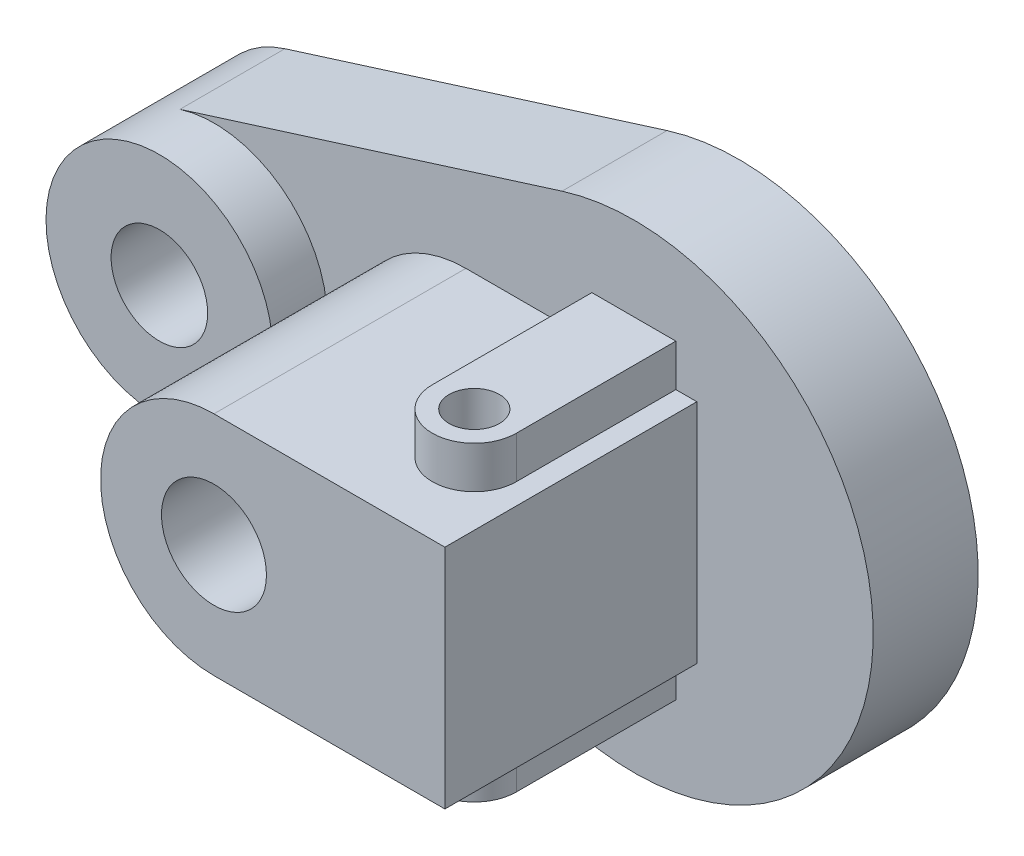
ISO-10303-21;
HEADER;
FILE_DESCRIPTION(('STEP AP214'),'2;1');
FILE_NAME('part.step','',(''),(''),'','','');
FILE_SCHEMA(('AUTOMOTIVE_DESIGN { 1 0 10303 214 1 1 1 1 }'));
ENDSEC;
DATA;
#1=APPLICATION_CONTEXT('core data for automotive mechanical design processes');
#2=APPLICATION_PROTOCOL_DEFINITION('international standard','automotive_design',2000,#1);
#3=PRODUCT_CONTEXT('',#1,'mechanical');
#4=PRODUCT('Part','Part','',(#3));
#5=PRODUCT_RELATED_PRODUCT_CATEGORY('part','',(#4));
#6=PRODUCT_DEFINITION_FORMATION('','',#4);
#7=PRODUCT_DEFINITION_CONTEXT('part definition',#1,'design');
#8=PRODUCT_DEFINITION('design','',#6,#7);
#9=PRODUCT_DEFINITION_SHAPE('','',#8);
#10=(LENGTH_UNIT() NAMED_UNIT(*) SI_UNIT(.MILLI.,.METRE.));
#11=(NAMED_UNIT(*) PLANE_ANGLE_UNIT() SI_UNIT($,.RADIAN.));
#12=(NAMED_UNIT(*) SI_UNIT($,.STERADIAN.) SOLID_ANGLE_UNIT());
#13=UNCERTAINTY_MEASURE_WITH_UNIT(LENGTH_MEASURE(1.E-05),#10,'distance_accuracy_value','');
#14=(GEOMETRIC_REPRESENTATION_CONTEXT(3) GLOBAL_UNCERTAINTY_ASSIGNED_CONTEXT((#13)) GLOBAL_UNIT_ASSIGNED_CONTEXT((#10,
#11,#12)) REPRESENTATION_CONTEXT('',''));
#15=CARTESIAN_POINT('',(0.,0.,0.));
#16=DIRECTION('',(0.,0.,1.));
#17=DIRECTION('',(1.,0.,0.));
#18=AXIS2_PLACEMENT_3D('',#15,#16,#17);
#19=CARTESIAN_POINT('',(0.,0.,25.));
#20=DIRECTION('',(0.,0.,1.));
#21=DIRECTION('',(1.,0.,0.));
#22=AXIS2_PLACEMENT_3D('',#19,#20,#21);
#23=PLANE('',#22);
#24=DIRECTION('',(0.,-1.,0.));
#25=VECTOR('',#24,1.);
#26=CARTESIAN_POINT('',(110.,37.,25.));
#27=LINE('',#26,#25);
#28=CARTESIAN_POINT('',(110.,37.,25.));
#29=VERTEX_POINT('',#28);
#30=CARTESIAN_POINT('',(110.,27.,25.));
#31=VERTEX_POINT('',#30);
#32=EDGE_CURVE('E164',#29,#31,#27,.T.);
#33=ORIENTED_EDGE('',*,*,#32,.T.);
#34=DIRECTION('',(-1.,0.,0.));
#35=VECTOR('',#34,1.);
#36=CARTESIAN_POINT('',(60.,27.,25.));
#37=LINE('',#36,#35);
#38=CARTESIAN_POINT('',(115.,27.,25.));
#39=VERTEX_POINT('',#38);
#40=EDGE_CURVE('E237',#39,#31,#37,.T.);
#41=ORIENTED_EDGE('',*,*,#40,.F.);
#42=DIRECTION('',(0.,1.,0.));
#43=VECTOR('',#42,1.);
#44=CARTESIAN_POINT('',(115.,27.,25.));
#45=LINE('',#44,#43);
#46=CARTESIAN_POINT('',(115.,-27.,25.));
#47=VERTEX_POINT('',#46);
#48=EDGE_CURVE('E248',#47,#39,#45,.T.);
#49=ORIENTED_EDGE('',*,*,#48,.F.);
#50=DIRECTION('',(1.,0.,0.));
#51=VECTOR('',#50,1.);
#52=CARTESIAN_POINT('',(115.,-27.,25.));
#53=LINE('',#52,#51);
#54=CARTESIAN_POINT('',(110.,-27.,25.));
#55=VERTEX_POINT('',#54);
#56=EDGE_CURVE('E242',#55,#47,#53,.T.);
#57=ORIENTED_EDGE('',*,*,#56,.F.);
#58=DIRECTION('',(0.,1.,0.));
#59=VECTOR('',#58,1.);
#60=CARTESIAN_POINT('',(110.,-37.,25.));
#61=LINE('',#60,#59);
#62=CARTESIAN_POINT('',(110.,-37.,25.));
#63=VERTEX_POINT('',#62);
#64=EDGE_CURVE('E220',#63,#55,#61,.T.);
#65=ORIENTED_EDGE('',*,*,#64,.F.);
#66=DIRECTION('',(1.,0.,0.));
#67=VECTOR('',#66,1.);
#68=CARTESIAN_POINT('',(90.,-37.,25.));
#69=LINE('',#68,#67);
#70=CARTESIAN_POINT('',(90.,-37.,25.));
#71=VERTEX_POINT('',#70);
#72=EDGE_CURVE('E65',#71,#63,#69,.T.);
#73=ORIENTED_EDGE('',*,*,#72,.F.);
#74=DIRECTION('',(0.,1.,0.));
#75=VECTOR('',#74,1.);
#76=CARTESIAN_POINT('',(90.,-37.,25.));
#77=LINE('',#76,#75);
#78=CARTESIAN_POINT('',(90.,-27.,25.));
#79=VERTEX_POINT('',#78);
#80=EDGE_CURVE('E219',#71,#79,#77,.T.);
#81=ORIENTED_EDGE('',*,*,#80,.T.);
#82=CARTESIAN_POINT('',(60.,-27.,25.));
#83=VERTEX_POINT('',#82);
#84=EDGE_CURVE('E246',#83,#79,#53,.T.);
#85=ORIENTED_EDGE('',*,*,#84,.F.);
#86=CARTESIAN_POINT('',(60.,0.,25.));
#87=DIRECTION('',(0.,0.,1.));
#88=DIRECTION('',(1.,0.,0.));
#89=AXIS2_PLACEMENT_3D('',#86,#87,#88);
#90=CIRCLE('',#89,27.);
#91=CARTESIAN_POINT('',(60.,27.,25.));
#92=VERTEX_POINT('',#91);
#93=EDGE_CURVE('E229',#92,#83,#90,.T.);
#94=ORIENTED_EDGE('',*,*,#93,.F.);
#95=CARTESIAN_POINT('',(90.,27.,25.));
#96=VERTEX_POINT('',#95);
#97=EDGE_CURVE('E252',#96,#92,#37,.T.);
#98=ORIENTED_EDGE('',*,*,#97,.F.);
#99=DIRECTION('',(0.,-1.,0.));
#100=VECTOR('',#99,1.);
#101=CARTESIAN_POINT('',(90.,37.,25.));
#102=LINE('',#101,#100);
#103=CARTESIAN_POINT('',(90.,37.,25.));
#104=VERTEX_POINT('',#103);
#105=EDGE_CURVE('E53',#104,#96,#102,.T.);
#106=ORIENTED_EDGE('',*,*,#105,.F.);
#107=DIRECTION('',(1.,0.,0.));
#108=VECTOR('',#107,1.);
#109=CARTESIAN_POINT('',(90.,37.,25.));
#110=LINE('',#109,#108);
#111=EDGE_CURVE('E180',#104,#29,#110,.T.);
#112=ORIENTED_EDGE('',*,*,#111,.T.);
#113=EDGE_LOOP('',(#33,#41,#49,#57,#65,#73,#81,#85,#94,#98,#106,#112));
#114=FACE_BOUND('',#113,.T.);
#115=CARTESIAN_POINT('',(0.,0.,25.));
#116=DIRECTION('',(0.,0.,-1.));
#117=DIRECTION('',(1.,0.,0.));
#118=AXIS2_PLACEMENT_3D('',#115,#116,#117);
#119=CIRCLE('',#118,27.);
#120=CARTESIAN_POINT('',(-8.1,25.7563584382575,25.));
#121=VERTEX_POINT('',#120);
#122=CARTESIAN_POINT('',(-8.1,-25.7563584382575,25.));
#123=VERTEX_POINT('',#122);
#124=EDGE_CURVE('E264',#121,#123,#119,.T.);
#125=ORIENTED_EDGE('',*,*,#124,.T.);
#126=DIRECTION('',(0.953939201416946,-0.3,0.));
#127=VECTOR('',#126,1.);
#128=CARTESIAN_POINT('',(-8.1,-25.7563584382575,25.));
#129=LINE('',#128,#127);
#130=CARTESIAN_POINT('',(82.9,-54.3745344807659,25.));
#131=VERTEX_POINT('',#130);
#132=EDGE_CURVE('E268',#123,#131,#129,.T.);
#133=ORIENTED_EDGE('',*,*,#132,.T.);
#134=CARTESIAN_POINT('',(100.,0.,25.));
#135=DIRECTION('',(0.,0.,1.));
#136=DIRECTION('',(1.,0.,0.));
#137=AXIS2_PLACEMENT_3D('',#134,#135,#136);
#138=CIRCLE('',#137,57.);
#139=CARTESIAN_POINT('',(82.9,54.3745344807659,25.));
#140=VERTEX_POINT('',#139);
#141=EDGE_CURVE('E271',#131,#140,#138,.T.);
#142=ORIENTED_EDGE('',*,*,#141,.T.);
#143=DIRECTION('',(-0.953939201416946,-0.3,0.));
#144=VECTOR('',#143,1.);
#145=CARTESIAN_POINT('',(-8.1,25.7563584382575,25.));
#146=LINE('',#145,#144);
#147=EDGE_CURVE('E272',#140,#121,#146,.T.);
#148=ORIENTED_EDGE('',*,*,#147,.T.);
#149=EDGE_LOOP('',(#125,#133,#142,#148));
#150=FACE_BOUND('',#149,.T.);
#151=ADVANCED_FACE('F39',(#114,#150),#23,.T.);
#152=CARTESIAN_POINT('',(0.,0.,38.));
#153=DIRECTION('',(0.,0.,-1.));
#154=DIRECTION('',(-1.,0.,0.));
#155=AXIS2_PLACEMENT_3D('',#152,#153,#154);
#156=CYLINDRICAL_SURFACE('',#155,27.);
#157=CARTESIAN_POINT('',(0.,0.,38.));
#158=DIRECTION('',(0.,0.,1.));
#159=DIRECTION('',(1.,0.,0.));
#160=AXIS2_PLACEMENT_3D('',#157,#158,#159);
#161=CIRCLE('',#160,27.);
#162=CARTESIAN_POINT('',(27.,0.,38.));
#163=VERTEX_POINT('',#162);
#164=EDGE_CURVE('E50',#163,#163,#161,.T.);
#165=ORIENTED_EDGE('',*,*,#164,.F.);
#166=EDGE_LOOP('',(#165));
#167=FACE_BOUND('',#166,.T.);
#168=DIRECTION('',(0.,0.,-1.));
#169=VECTOR('',#168,1.);
#170=CARTESIAN_POINT('',(-8.1,-25.7563584382575,25.));
#171=LINE('',#170,#169);
#172=CARTESIAN_POINT('',(-8.1,-25.7563584382575,0.));
#173=VERTEX_POINT('',#172);
#174=EDGE_CURVE('E289',#123,#173,#171,.T.);
#175=ORIENTED_EDGE('',*,*,#174,.F.);
#176=ORIENTED_EDGE('',*,*,#124,.F.);
#177=DIRECTION('',(0.,0.,-1.));
#178=VECTOR('',#177,1.);
#179=CARTESIAN_POINT('',(-8.1,25.7563584382575,25.));
#180=LINE('',#179,#178);
#181=CARTESIAN_POINT('',(-8.1,25.7563584382575,0.));
#182=VERTEX_POINT('',#181);
#183=EDGE_CURVE('E277',#121,#182,#180,.T.);
#184=ORIENTED_EDGE('',*,*,#183,.T.);
#185=CARTESIAN_POINT('',(0.,0.,0.));
#186=DIRECTION('',(0.,0.,1.));
#187=DIRECTION('',(1.,0.,0.));
#188=AXIS2_PLACEMENT_3D('',#185,#186,#187);
#189=CIRCLE('',#188,27.);
#190=EDGE_CURVE('E300',#182,#173,#189,.T.);
#191=ORIENTED_EDGE('',*,*,#190,.T.);
#192=EDGE_LOOP('',(#175,#176,#184,#191));
#193=FACE_BOUND('',#192,.T.);
#194=ADVANCED_FACE('F41',(#167,#193),#156,.T.);
#195=CARTESIAN_POINT('',(0.,0.,38.));
#196=DIRECTION('',(0.,0.,1.));
#197=DIRECTION('',(1.,0.,0.));
#198=AXIS2_PLACEMENT_3D('',#195,#196,#197);
#199=PLANE('',#198);
#200=ORIENTED_EDGE('',*,*,#164,.T.);
#201=EDGE_LOOP('',(#200));
#202=FACE_BOUND('',#201,.T.);
#203=CARTESIAN_POINT('',(0.,0.,38.));
#204=DIRECTION('',(0.,0.,1.));
#205=DIRECTION('',(1.,0.,0.));
#206=AXIS2_PLACEMENT_3D('',#203,#204,#205);
#207=CIRCLE('',#206,11.5);
#208=CARTESIAN_POINT('',(11.5,0.,38.));
#209=VERTEX_POINT('',#208);
#210=EDGE_CURVE('E294',#209,#209,#207,.T.);
#211=ORIENTED_EDGE('',*,*,#210,.F.);
#212=EDGE_LOOP('',(#211));
#213=FACE_BOUND('',#212,.T.);
#214=ADVANCED_FACE('F336',(#202,#213),#199,.T.);
#215=CARTESIAN_POINT('',(0.,0.,0.));
#216=DIRECTION('',(0.,0.,1.));
#217=DIRECTION('',(1.,0.,0.));
#218=AXIS2_PLACEMENT_3D('',#215,#216,#217);
#219=PLANE('',#218);
#220=ORIENTED_EDGE('',*,*,#190,.F.);
#221=DIRECTION('',(-0.953939201416946,-0.3,0.));
#222=VECTOR('',#221,1.);
#223=CARTESIAN_POINT('',(-8.1,25.7563584382575,0.));
#224=LINE('',#223,#222);
#225=CARTESIAN_POINT('',(82.9,54.3745344807659,0.));
#226=VERTEX_POINT('',#225);
#227=EDGE_CURVE('E267',#226,#182,#224,.T.);
#228=ORIENTED_EDGE('',*,*,#227,.F.);
#229=CARTESIAN_POINT('',(100.,0.,0.));
#230=DIRECTION('',(0.,0.,1.));
#231=DIRECTION('',(1.,0.,0.));
#232=AXIS2_PLACEMENT_3D('',#229,#230,#231);
#233=CIRCLE('',#232,57.);
#234=CARTESIAN_POINT('',(82.9,-54.3745344807659,0.));
#235=VERTEX_POINT('',#234);
#236=EDGE_CURVE('E279',#235,#226,#233,.T.);
#237=ORIENTED_EDGE('',*,*,#236,.F.);
#238=DIRECTION('',(0.953939201416946,-0.3,0.));
#239=VECTOR('',#238,1.);
#240=CARTESIAN_POINT('',(-8.1,-25.7563584382575,0.));
#241=LINE('',#240,#239);
#242=EDGE_CURVE('E262',#173,#235,#241,.T.);
#243=ORIENTED_EDGE('',*,*,#242,.F.);
#244=EDGE_LOOP('',(#220,#228,#237,#243));
#245=FACE_BOUND('',#244,.T.);
#246=CARTESIAN_POINT('',(0.,0.,0.));
#247=DIRECTION('',(0.,0.,1.));
#248=DIRECTION('',(1.,0.,0.));
#249=AXIS2_PLACEMENT_3D('',#246,#247,#248);
#250=CIRCLE('',#249,11.5);
#251=CARTESIAN_POINT('',(11.5,0.,0.));
#252=VERTEX_POINT('',#251);
#253=EDGE_CURVE('E291',#252,#252,#250,.T.);
#254=ORIENTED_EDGE('',*,*,#253,.T.);
#255=EDGE_LOOP('',(#254));
#256=FACE_BOUND('',#255,.T.);
#257=ADVANCED_FACE('F306',(#245,#256),#219,.F.);
#258=CARTESIAN_POINT('',(0.,0.,38.));
#259=DIRECTION('',(0.,0.,-1.));
#260=DIRECTION('',(-1.,0.,0.));
#261=AXIS2_PLACEMENT_3D('',#258,#259,#260);
#262=CYLINDRICAL_SURFACE('',#261,11.5);
#263=ORIENTED_EDGE('',*,*,#210,.T.);
#264=EDGE_LOOP('',(#263));
#265=FACE_BOUND('',#264,.T.);
#266=ORIENTED_EDGE('',*,*,#253,.F.);
#267=EDGE_LOOP('',(#266));
#268=FACE_BOUND('',#267,.T.);
#269=ADVANCED_FACE('F328',(#265,#268),#262,.F.);
#270=CARTESIAN_POINT('',(-8.1,-25.7563584382575,25.));
#271=DIRECTION('',(0.3,0.953939201416946,0.));
#272=DIRECTION('',(-0.953939201416946,0.3,0.));
#273=AXIS2_PLACEMENT_3D('',#270,#271,#272);
#274=PLANE('',#273);
#275=ORIENTED_EDGE('',*,*,#242,.T.);
#276=DIRECTION('',(0.,0.,-1.));
#277=VECTOR('',#276,1.);
#278=CARTESIAN_POINT('',(82.9,-54.3745344807659,25.));
#279=LINE('',#278,#277);
#280=EDGE_CURVE('E290',#131,#235,#279,.T.);
#281=ORIENTED_EDGE('',*,*,#280,.F.);
#282=ORIENTED_EDGE('',*,*,#132,.F.);
#283=ORIENTED_EDGE('',*,*,#174,.T.);
#284=EDGE_LOOP('',(#275,#281,#282,#283));
#285=FACE_BOUND('',#284,.T.);
#286=ADVANCED_FACE('F315',(#285),#274,.F.);
#287=CARTESIAN_POINT('',(100.,0.,25.));
#288=DIRECTION('',(0.,0.,-1.));
#289=DIRECTION('',(-1.,0.,0.));
#290=AXIS2_PLACEMENT_3D('',#287,#288,#289);
#291=CYLINDRICAL_SURFACE('',#290,57.);
#292=ORIENTED_EDGE('',*,*,#236,.T.);
#293=DIRECTION('',(0.,0.,-1.));
#294=VECTOR('',#293,1.);
#295=CARTESIAN_POINT('',(82.9,54.3745344807659,25.));
#296=LINE('',#295,#294);
#297=EDGE_CURVE('E284',#140,#226,#296,.T.);
#298=ORIENTED_EDGE('',*,*,#297,.F.);
#299=ORIENTED_EDGE('',*,*,#141,.F.);
#300=ORIENTED_EDGE('',*,*,#280,.T.);
#301=EDGE_LOOP('',(#292,#298,#299,#300));
#302=FACE_BOUND('',#301,.T.);
#303=ADVANCED_FACE('F319',(#302),#291,.T.);
#304=CARTESIAN_POINT('',(-8.1,25.7563584382575,25.));
#305=DIRECTION('',(0.3,-0.953939201416946,0.));
#306=DIRECTION('',(0.953939201416946,0.3,0.));
#307=AXIS2_PLACEMENT_3D('',#304,#305,#306);
#308=PLANE('',#307);
#309=ORIENTED_EDGE('',*,*,#227,.T.);
#310=ORIENTED_EDGE('',*,*,#183,.F.);
#311=ORIENTED_EDGE('',*,*,#147,.F.);
#312=ORIENTED_EDGE('',*,*,#297,.T.);
#313=EDGE_LOOP('',(#309,#310,#311,#312));
#314=FACE_BOUND('',#313,.T.);
#315=ADVANCED_FACE('F318',(#314),#308,.F.);
#316=CARTESIAN_POINT('',(60.,0.,85.));
#317=DIRECTION('',(0.,0.,-1.));
#318=DIRECTION('',(-1.,0.,0.));
#319=AXIS2_PLACEMENT_3D('',#316,#317,#318);
#320=CYLINDRICAL_SURFACE('',#319,27.);
#321=ORIENTED_EDGE('',*,*,#93,.T.);
#322=DIRECTION('',(0.,0.,-1.));
#323=VECTOR('',#322,1.);
#324=CARTESIAN_POINT('',(60.,-27.,85.));
#325=LINE('',#324,#323);
#326=CARTESIAN_POINT('',(60.,-27.,85.));
#327=VERTEX_POINT('',#326);
#328=EDGE_CURVE('E265',#327,#83,#325,.T.);
#329=ORIENTED_EDGE('',*,*,#328,.F.);
#330=CARTESIAN_POINT('',(60.,0.,85.));
#331=DIRECTION('',(0.,0.,1.));
#332=DIRECTION('',(1.,0.,0.));
#333=AXIS2_PLACEMENT_3D('',#330,#331,#332);
#334=CIRCLE('',#333,27.);
#335=CARTESIAN_POINT('',(60.,27.,85.));
#336=VERTEX_POINT('',#335);
#337=EDGE_CURVE('E235',#336,#327,#334,.T.);
#338=ORIENTED_EDGE('',*,*,#337,.F.);
#339=DIRECTION('',(0.,0.,-1.));
#340=VECTOR('',#339,1.);
#341=CARTESIAN_POINT('',(60.,27.,85.));
#342=LINE('',#341,#340);
#343=EDGE_CURVE('E245',#336,#92,#342,.T.);
#344=ORIENTED_EDGE('',*,*,#343,.T.);
#345=EDGE_LOOP('',(#321,#329,#338,#344));
#346=FACE_BOUND('',#345,.T.);
#347=ADVANCED_FACE('F330',(#346),#320,.T.);
#348=CARTESIAN_POINT('',(115.,-27.,85.));
#349=DIRECTION('',(0.,1.,0.));
#350=DIRECTION('',(0.,0.,1.));
#351=AXIS2_PLACEMENT_3D('',#348,#349,#350);
#352=PLANE('',#351);
#353=DIRECTION('',(0.,0.,-1.));
#354=VECTOR('',#353,1.);
#355=CARTESIAN_POINT('',(90.,-27.,63.));
#356=LINE('',#355,#354);
#357=CARTESIAN_POINT('',(90.,-27.,63.));
#358=VERTEX_POINT('',#357);
#359=EDGE_CURVE('E209',#358,#79,#356,.T.);
#360=ORIENTED_EDGE('',*,*,#359,.F.);
#361=CARTESIAN_POINT('',(100.,-27.,63.));
#362=DIRECTION('',(0.,-1.,0.));
#363=DIRECTION('',(0.,0.,-1.));
#364=AXIS2_PLACEMENT_3D('',#361,#362,#363);
#365=CIRCLE('',#364,10.);
#366=CARTESIAN_POINT('',(110.,-27.,63.));
#367=VERTEX_POINT('',#366);
#368=EDGE_CURVE('E194',#367,#358,#365,.T.);
#369=ORIENTED_EDGE('',*,*,#368,.F.);
#370=DIRECTION('',(0.,0.,1.));
#371=VECTOR('',#370,1.);
#372=CARTESIAN_POINT('',(110.,-27.,25.));
#373=LINE('',#372,#371);
#374=EDGE_CURVE('E205',#55,#367,#373,.T.);
#375=ORIENTED_EDGE('',*,*,#374,.F.);
#376=ORIENTED_EDGE('',*,*,#56,.T.);
#377=DIRECTION('',(0.,0.,-1.));
#378=VECTOR('',#377,1.);
#379=CARTESIAN_POINT('',(115.,-27.,85.));
#380=LINE('',#379,#378);
#381=CARTESIAN_POINT('',(115.,-27.,85.));
#382=VERTEX_POINT('',#381);
#383=EDGE_CURVE('E259',#382,#47,#380,.T.);
#384=ORIENTED_EDGE('',*,*,#383,.F.);
#385=DIRECTION('',(1.,0.,0.));
#386=VECTOR('',#385,1.);
#387=CARTESIAN_POINT('',(115.,-27.,85.));
#388=LINE('',#387,#386);
#389=EDGE_CURVE('E234',#327,#382,#388,.T.);
#390=ORIENTED_EDGE('',*,*,#389,.F.);
#391=ORIENTED_EDGE('',*,*,#328,.T.);
#392=ORIENTED_EDGE('',*,*,#84,.T.);
#393=EDGE_LOOP('',(#360,#369,#375,#376,#384,#390,#391,#392));
#394=FACE_BOUND('',#393,.T.);
#395=ADVANCED_FACE('F342',(#394),#352,.F.);
#396=CARTESIAN_POINT('',(115.,27.,85.));
#397=DIRECTION('',(-1.,0.,0.));
#398=DIRECTION('',(0.,0.,1.));
#399=AXIS2_PLACEMENT_3D('',#396,#397,#398);
#400=PLANE('',#399);
#401=ORIENTED_EDGE('',*,*,#48,.T.);
#402=DIRECTION('',(0.,0.,-1.));
#403=VECTOR('',#402,1.);
#404=CARTESIAN_POINT('',(115.,27.,85.));
#405=LINE('',#404,#403);
#406=CARTESIAN_POINT('',(115.,27.,85.));
#407=VERTEX_POINT('',#406);
#408=EDGE_CURVE('E260',#407,#39,#405,.T.);
#409=ORIENTED_EDGE('',*,*,#408,.F.);
#410=DIRECTION('',(0.,1.,0.));
#411=VECTOR('',#410,1.);
#412=CARTESIAN_POINT('',(115.,27.,85.));
#413=LINE('',#412,#411);
#414=EDGE_CURVE('E236',#382,#407,#413,.T.);
#415=ORIENTED_EDGE('',*,*,#414,.F.);
#416=ORIENTED_EDGE('',*,*,#383,.T.);
#417=EDGE_LOOP('',(#401,#409,#415,#416));
#418=FACE_BOUND('',#417,.T.);
#419=ADVANCED_FACE('F350',(#418),#400,.F.);
#420=CARTESIAN_POINT('',(60.,27.,85.));
#421=DIRECTION('',(0.,-1.,0.));
#422=DIRECTION('',(0.,0.,-1.));
#423=AXIS2_PLACEMENT_3D('',#420,#421,#422);
#424=PLANE('',#423);
#425=ORIENTED_EDGE('',*,*,#40,.T.);
#426=DIRECTION('',(0.,0.,1.));
#427=VECTOR('',#426,1.);
#428=CARTESIAN_POINT('',(110.,27.,25.));
#429=LINE('',#428,#427);
#430=CARTESIAN_POINT('',(110.,27.,63.));
#431=VERTEX_POINT('',#430);
#432=EDGE_CURVE('E183',#31,#431,#429,.T.);
#433=ORIENTED_EDGE('',*,*,#432,.T.);
#434=CARTESIAN_POINT('',(100.,27.,63.));
#435=DIRECTION('',(0.,-1.,0.));
#436=DIRECTION('',(0.,0.,-1.));
#437=AXIS2_PLACEMENT_3D('',#434,#435,#436);
#438=CIRCLE('',#437,10.);
#439=CARTESIAN_POINT('',(90.,27.,63.));
#440=VERTEX_POINT('',#439);
#441=EDGE_CURVE('E159',#431,#440,#438,.T.);
#442=ORIENTED_EDGE('',*,*,#441,.T.);
#443=DIRECTION('',(0.,0.,-1.));
#444=VECTOR('',#443,1.);
#445=CARTESIAN_POINT('',(90.,27.,63.));
#446=LINE('',#445,#444);
#447=EDGE_CURVE('E171',#440,#96,#446,.T.);
#448=ORIENTED_EDGE('',*,*,#447,.T.);
#449=ORIENTED_EDGE('',*,*,#97,.T.);
#450=ORIENTED_EDGE('',*,*,#343,.F.);
#451=DIRECTION('',(-1.,0.,0.));
#452=VECTOR('',#451,1.);
#453=CARTESIAN_POINT('',(60.,27.,85.));
#454=LINE('',#453,#452);
#455=EDGE_CURVE('E238',#407,#336,#454,.T.);
#456=ORIENTED_EDGE('',*,*,#455,.F.);
#457=ORIENTED_EDGE('',*,*,#408,.T.);
#458=EDGE_LOOP('',(#425,#433,#442,#448,#449,#450,#456,#457));
#459=FACE_BOUND('',#458,.T.);
#460=ADVANCED_FACE('F355',(#459),#424,.F.);
#461=CARTESIAN_POINT('',(60.,0.,85.));
#462=DIRECTION('',(0.,0.,1.));
#463=DIRECTION('',(1.,0.,0.));
#464=AXIS2_PLACEMENT_3D('',#461,#462,#463);
#465=PLANE('',#464);
#466=CARTESIAN_POINT('',(60.,0.,85.));
#467=DIRECTION('',(0.,0.,1.));
#468=DIRECTION('',(1.,0.,0.));
#469=AXIS2_PLACEMENT_3D('',#466,#467,#468);
#470=CIRCLE('',#469,12.5);
#471=CARTESIAN_POINT('',(72.5,0.,85.));
#472=VERTEX_POINT('',#471);
#473=EDGE_CURVE('E223',#472,#472,#470,.T.);
#474=ORIENTED_EDGE('',*,*,#473,.F.);
#475=EDGE_LOOP('',(#474));
#476=FACE_BOUND('',#475,.T.);
#477=ORIENTED_EDGE('',*,*,#337,.T.);
#478=ORIENTED_EDGE('',*,*,#389,.T.);
#479=ORIENTED_EDGE('',*,*,#414,.T.);
#480=ORIENTED_EDGE('',*,*,#455,.T.);
#481=EDGE_LOOP('',(#477,#478,#479,#480));
#482=FACE_BOUND('',#481,.T.);
#483=ADVANCED_FACE('F352',(#476,#482),#465,.T.);
#484=CARTESIAN_POINT('',(60.,0.,25.));
#485=DIRECTION('',(0.,0.,1.));
#486=DIRECTION('',(1.,0.,0.));
#487=AXIS2_PLACEMENT_3D('',#484,#485,#486);
#488=CYLINDRICAL_SURFACE('',#487,12.5);
#489=CARTESIAN_POINT('',(60.,0.,25.));
#490=DIRECTION('',(0.,0.,1.));
#491=DIRECTION('',(1.,0.,0.));
#492=AXIS2_PLACEMENT_3D('',#489,#490,#491);
#493=CIRCLE('',#492,12.5);
#494=CARTESIAN_POINT('',(72.5,0.,25.));
#495=VERTEX_POINT('',#494);
#496=EDGE_CURVE('E228',#495,#495,#493,.T.);
#497=ORIENTED_EDGE('',*,*,#496,.F.);
#498=EDGE_LOOP('',(#497));
#499=FACE_BOUND('',#498,.T.);
#500=ORIENTED_EDGE('',*,*,#473,.T.);
#501=EDGE_LOOP('',(#500));
#502=FACE_BOUND('',#501,.T.);
#503=ADVANCED_FACE('F359',(#499,#502),#488,.F.);
#504=CARTESIAN_POINT('',(60.,0.,25.));
#505=DIRECTION('',(0.,0.,1.));
#506=DIRECTION('',(1.,0.,0.));
#507=AXIS2_PLACEMENT_3D('',#504,#505,#506);
#508=PLANE('',#507);
#509=ORIENTED_EDGE('',*,*,#496,.T.);
#510=EDGE_LOOP('',(#509));
#511=FACE_BOUND('',#510,.T.);
#512=ADVANCED_FACE('F365',(#511),#508,.T.);
#513=CARTESIAN_POINT('',(100.,-37.,63.));
#514=DIRECTION('',(0.,-1.,0.));
#515=DIRECTION('',(0.,0.,-1.));
#516=AXIS2_PLACEMENT_3D('',#513,#514,#515);
#517=PLANE('',#516);
#518=CARTESIAN_POINT('',(100.,-37.,63.));
#519=DIRECTION('',(0.,-1.,0.));
#520=DIRECTION('',(0.,0.,-1.));
#521=AXIS2_PLACEMENT_3D('',#518,#519,#520);
#522=CIRCLE('',#521,10.);
#523=CARTESIAN_POINT('',(110.,-37.,63.));
#524=VERTEX_POINT('',#523);
#525=CARTESIAN_POINT('',(90.,-37.,63.));
#526=VERTEX_POINT('',#525);
#527=EDGE_CURVE('E196',#524,#526,#522,.T.);
#528=ORIENTED_EDGE('',*,*,#527,.T.);
#529=DIRECTION('',(0.,0.,-1.));
#530=VECTOR('',#529,1.);
#531=CARTESIAN_POINT('',(90.,-37.,63.));
#532=LINE('',#531,#530);
#533=EDGE_CURVE('E203',#526,#71,#532,.T.);
#534=ORIENTED_EDGE('',*,*,#533,.T.);
#535=ORIENTED_EDGE('',*,*,#72,.T.);
#536=DIRECTION('',(0.,0.,1.));
#537=VECTOR('',#536,1.);
#538=CARTESIAN_POINT('',(110.,-37.,25.));
#539=LINE('',#538,#537);
#540=EDGE_CURVE('E202',#63,#524,#539,.T.);
#541=ORIENTED_EDGE('',*,*,#540,.T.);
#542=EDGE_LOOP('',(#528,#534,#535,#541));
#543=FACE_BOUND('',#542,.T.);
#544=CARTESIAN_POINT('',(100.,-37.,63.));
#545=DIRECTION('',(0.,-1.,0.));
#546=DIRECTION('',(0.,0.,-1.));
#547=AXIS2_PLACEMENT_3D('',#544,#545,#546);
#548=CIRCLE('',#547,6.);
#549=CARTESIAN_POINT('',(100.,-37.,57.));
#550=VERTEX_POINT('',#549);
#551=EDGE_CURVE('E195',#550,#550,#548,.T.);
#552=ORIENTED_EDGE('',*,*,#551,.F.);
#553=EDGE_LOOP('',(#552));
#554=FACE_BOUND('',#553,.T.);
#555=ADVANCED_FACE('F366',(#543,#554),#517,.T.);
#556=CARTESIAN_POINT('',(100.,-37.,63.));
#557=DIRECTION('',(0.,1.,0.));
#558=DIRECTION('',(0.,0.,1.));
#559=AXIS2_PLACEMENT_3D('',#556,#557,#558);
#560=CYLINDRICAL_SURFACE('',#559,10.);
#561=ORIENTED_EDGE('',*,*,#368,.T.);
#562=DIRECTION('',(0.,1.,0.));
#563=VECTOR('',#562,1.);
#564=CARTESIAN_POINT('',(90.,-37.,63.));
#565=LINE('',#564,#563);
#566=EDGE_CURVE('E225',#526,#358,#565,.T.);
#567=ORIENTED_EDGE('',*,*,#566,.F.);
#568=ORIENTED_EDGE('',*,*,#527,.F.);
#569=DIRECTION('',(0.,1.,0.));
#570=VECTOR('',#569,1.);
#571=CARTESIAN_POINT('',(110.,-37.,63.));
#572=LINE('',#571,#570);
#573=EDGE_CURVE('E210',#524,#367,#572,.T.);
#574=ORIENTED_EDGE('',*,*,#573,.T.);
#575=EDGE_LOOP('',(#561,#567,#568,#574));
#576=FACE_BOUND('',#575,.T.);
#577=ADVANCED_FACE('F367',(#576),#560,.T.);
#578=CARTESIAN_POINT('',(90.,-37.,63.));
#579=DIRECTION('',(1.,0.,0.));
#580=DIRECTION('',(0.,0.,-1.));
#581=AXIS2_PLACEMENT_3D('',#578,#579,#580);
#582=PLANE('',#581);
#583=ORIENTED_EDGE('',*,*,#359,.T.);
#584=ORIENTED_EDGE('',*,*,#80,.F.);
#585=ORIENTED_EDGE('',*,*,#533,.F.);
#586=ORIENTED_EDGE('',*,*,#566,.T.);
#587=EDGE_LOOP('',(#583,#584,#585,#586));
#588=FACE_BOUND('',#587,.T.);
#589=ADVANCED_FACE('F373',(#588),#582,.F.);
#590=CARTESIAN_POINT('',(110.,-37.,25.));
#591=DIRECTION('',(-1.,0.,0.));
#592=DIRECTION('',(0.,0.,1.));
#593=AXIS2_PLACEMENT_3D('',#590,#591,#592);
#594=PLANE('',#593);
#595=ORIENTED_EDGE('',*,*,#374,.T.);
#596=ORIENTED_EDGE('',*,*,#573,.F.);
#597=ORIENTED_EDGE('',*,*,#540,.F.);
#598=ORIENTED_EDGE('',*,*,#64,.T.);
#599=EDGE_LOOP('',(#595,#596,#597,#598));
#600=FACE_BOUND('',#599,.T.);
#601=ADVANCED_FACE('F380',(#600),#594,.F.);
#602=CARTESIAN_POINT('',(100.,-37.,63.));
#603=DIRECTION('',(0.,1.,0.));
#604=DIRECTION('',(0.,0.,1.));
#605=AXIS2_PLACEMENT_3D('',#602,#603,#604);
#606=CYLINDRICAL_SURFACE('',#605,6.);
#607=ORIENTED_EDGE('',*,*,#551,.T.);
#608=EDGE_LOOP('',(#607));
#609=FACE_BOUND('',#608,.T.);
#610=CARTESIAN_POINT('',(100.,-27.,63.));
#611=DIRECTION('',(0.,-1.,0.));
#612=DIRECTION('',(0.,0.,-1.));
#613=AXIS2_PLACEMENT_3D('',#610,#611,#612);
#614=CIRCLE('',#613,6.);
#615=CARTESIAN_POINT('',(100.,-27.,57.));
#616=VERTEX_POINT('',#615);
#617=EDGE_CURVE('E163',#616,#616,#614,.T.);
#618=ORIENTED_EDGE('',*,*,#617,.F.);
#619=EDGE_LOOP('',(#618));
#620=FACE_BOUND('',#619,.T.);
#621=ADVANCED_FACE('F381',(#609,#620),#606,.F.);
#622=ORIENTED_EDGE('',*,*,#617,.T.);
#623=EDGE_LOOP('',(#622));
#624=FACE_BOUND('',#623,.T.);
#625=ADVANCED_FACE('F349',(#624),#352,.F.);
#626=CARTESIAN_POINT('',(100.,37.,63.));
#627=DIRECTION('',(0.,-1.,0.));
#628=DIRECTION('',(0.,0.,-1.));
#629=AXIS2_PLACEMENT_3D('',#626,#627,#628);
#630=CYLINDRICAL_SURFACE('',#629,10.);
#631=ORIENTED_EDGE('',*,*,#441,.F.);
#632=DIRECTION('',(0.,-1.,0.));
#633=VECTOR('',#632,1.);
#634=CARTESIAN_POINT('',(110.,37.,63.));
#635=LINE('',#634,#633);
#636=CARTESIAN_POINT('',(110.,37.,63.));
#637=VERTEX_POINT('',#636);
#638=EDGE_CURVE('E152',#637,#431,#635,.T.);
#639=ORIENTED_EDGE('',*,*,#638,.F.);
#640=CARTESIAN_POINT('',(100.,37.,63.));
#641=DIRECTION('',(0.,-1.,0.));
#642=DIRECTION('',(0.,0.,-1.));
#643=AXIS2_PLACEMENT_3D('',#640,#641,#642);
#644=CIRCLE('',#643,10.);
#645=CARTESIAN_POINT('',(90.,37.,63.));
#646=VERTEX_POINT('',#645);
#647=EDGE_CURVE('E160',#637,#646,#644,.T.);
#648=ORIENTED_EDGE('',*,*,#647,.T.);
#649=DIRECTION('',(0.,-1.,0.));
#650=VECTOR('',#649,1.);
#651=CARTESIAN_POINT('',(90.,37.,63.));
#652=LINE('',#651,#650);
#653=EDGE_CURVE('E181',#646,#440,#652,.T.);
#654=ORIENTED_EDGE('',*,*,#653,.T.);
#655=EDGE_LOOP('',(#631,#639,#648,#654));
#656=FACE_BOUND('',#655,.T.);
#657=ADVANCED_FACE('F156',(#656),#630,.T.);
#658=CARTESIAN_POINT('',(110.,37.,25.));
#659=DIRECTION('',(1.,0.,0.));
#660=DIRECTION('',(0.,0.,-1.));
#661=AXIS2_PLACEMENT_3D('',#658,#659,#660);
#662=PLANE('',#661);
#663=ORIENTED_EDGE('',*,*,#432,.F.);
#664=ORIENTED_EDGE('',*,*,#32,.F.);
#665=DIRECTION('',(0.,0.,1.));
#666=VECTOR('',#665,1.);
#667=CARTESIAN_POINT('',(110.,37.,25.));
#668=LINE('',#667,#666);
#669=EDGE_CURVE('E168',#29,#637,#668,.T.);
#670=ORIENTED_EDGE('',*,*,#669,.T.);
#671=ORIENTED_EDGE('',*,*,#638,.T.);
#672=EDGE_LOOP('',(#663,#664,#670,#671));
#673=FACE_BOUND('',#672,.T.);
#674=ADVANCED_FACE('F172',(#673),#662,.T.);
#675=CARTESIAN_POINT('',(90.,37.,63.));
#676=DIRECTION('',(-1.,0.,0.));
#677=DIRECTION('',(0.,0.,1.));
#678=AXIS2_PLACEMENT_3D('',#675,#676,#677);
#679=PLANE('',#678);
#680=ORIENTED_EDGE('',*,*,#447,.F.);
#681=ORIENTED_EDGE('',*,*,#653,.F.);
#682=DIRECTION('',(0.,0.,-1.));
#683=VECTOR('',#682,1.);
#684=CARTESIAN_POINT('',(90.,37.,63.));
#685=LINE('',#684,#683);
#686=EDGE_CURVE('E175',#646,#104,#685,.T.);
#687=ORIENTED_EDGE('',*,*,#686,.T.);
#688=ORIENTED_EDGE('',*,*,#105,.T.);
#689=EDGE_LOOP('',(#680,#681,#687,#688));
#690=FACE_BOUND('',#689,.T.);
#691=ADVANCED_FACE('F391',(#690),#679,.T.);
#692=CARTESIAN_POINT('',(100.,37.,63.));
#693=DIRECTION('',(0.,1.,0.));
#694=DIRECTION('',(0.,0.,-1.));
#695=AXIS2_PLACEMENT_3D('',#692,#693,#694);
#696=PLANE('',#695);
#697=CARTESIAN_POINT('',(100.,37.,63.));
#698=DIRECTION('',(0.,-1.,0.));
#699=DIRECTION('',(0.,0.,-1.));
#700=AXIS2_PLACEMENT_3D('',#697,#698,#699);
#701=CIRCLE('',#700,6.);
#702=CARTESIAN_POINT('',(100.,37.,57.));
#703=VERTEX_POINT('',#702);
#704=EDGE_CURVE('E188',#703,#703,#701,.T.);
#705=ORIENTED_EDGE('',*,*,#704,.T.);
#706=EDGE_LOOP('',(#705));
#707=FACE_BOUND('',#706,.T.);
#708=ORIENTED_EDGE('',*,*,#647,.F.);
#709=ORIENTED_EDGE('',*,*,#669,.F.);
#710=ORIENTED_EDGE('',*,*,#111,.F.);
#711=ORIENTED_EDGE('',*,*,#686,.F.);
#712=EDGE_LOOP('',(#708,#709,#710,#711));
#713=FACE_BOUND('',#712,.T.);
#714=ADVANCED_FACE('F166',(#707,#713),#696,.T.);
#715=CARTESIAN_POINT('',(100.,37.,63.));
#716=DIRECTION('',(0.,-1.,0.));
#717=DIRECTION('',(0.,0.,-1.));
#718=AXIS2_PLACEMENT_3D('',#715,#716,#717);
#719=CYLINDRICAL_SURFACE('',#718,6.);
#720=ORIENTED_EDGE('',*,*,#704,.F.);
#721=EDGE_LOOP('',(#720));
#722=FACE_BOUND('',#721,.T.);
#723=CARTESIAN_POINT('',(100.,27.,63.));
#724=DIRECTION('',(0.,-1.,0.));
#725=DIRECTION('',(0.,0.,-1.));
#726=AXIS2_PLACEMENT_3D('',#723,#724,#725);
#727=CIRCLE('',#726,6.);
#728=CARTESIAN_POINT('',(100.,27.,57.));
#729=VERTEX_POINT('',#728);
#730=EDGE_CURVE('E11',#729,#729,#727,.T.);
#731=ORIENTED_EDGE('',*,*,#730,.T.);
#732=EDGE_LOOP('',(#731));
#733=FACE_BOUND('',#732,.T.);
#734=ADVANCED_FACE('F397',(#722,#733),#719,.F.);
#735=ORIENTED_EDGE('',*,*,#730,.F.);
#736=EDGE_LOOP('',(#735));
#737=FACE_BOUND('',#736,.T.);
#738=ADVANCED_FACE('F360',(#737),#424,.F.);
#739=CLOSED_SHELL('',(#151,#194,#214,#257,#269,#286,#303,#315,#347,#395,#419,#460,#483,#503,
#512,#555,#577,#589,#601,#621,#625,#657,#674,#691,#714,#734,#738));
#740=MANIFOLD_SOLID_BREP('B2',#739);
#741=ADVANCED_BREP_SHAPE_REPRESENTATION('',(#18,#740),#14);
#742=SHAPE_DEFINITION_REPRESENTATION(#9,#741);
ENDSEC;
END-ISO-10303-21;
